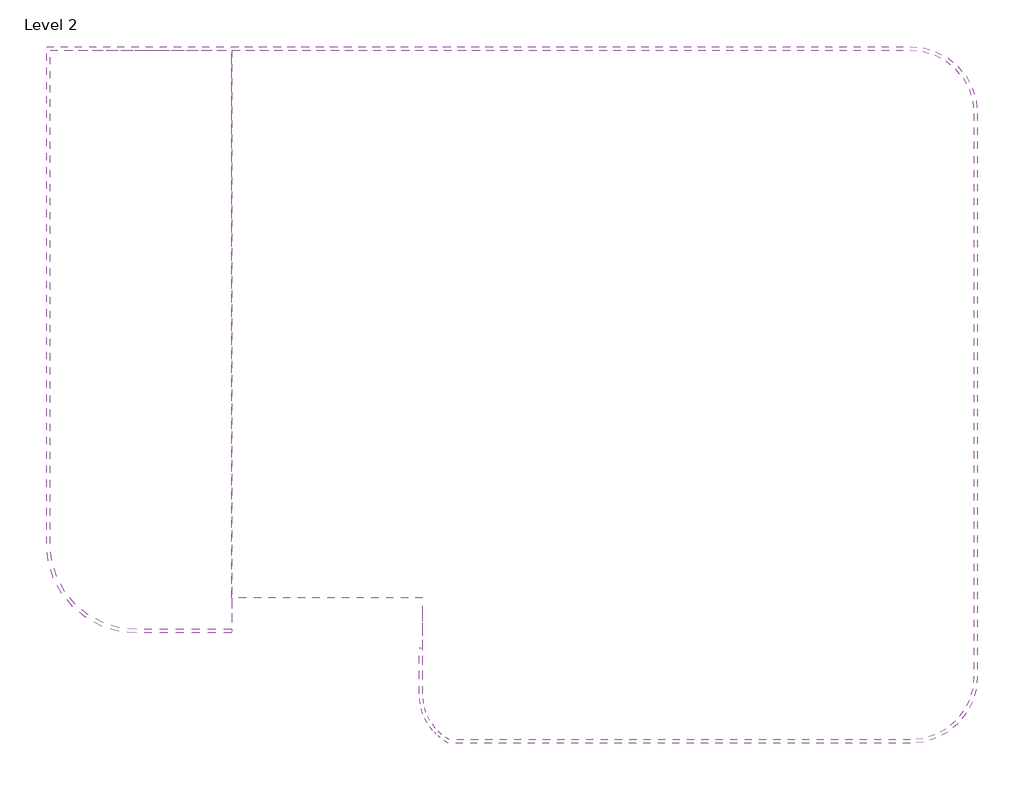
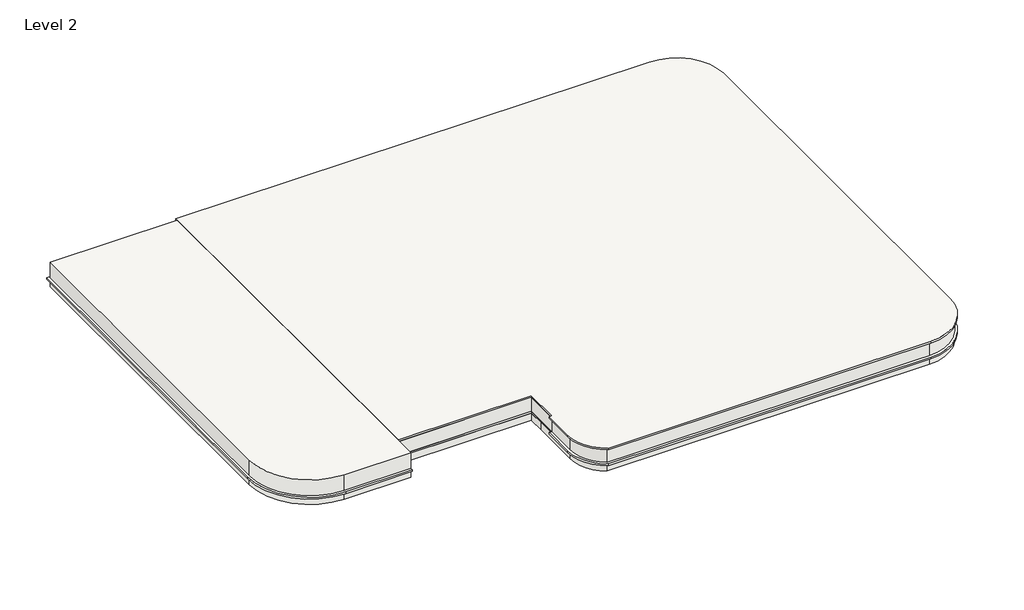
# One storey: 5 slabs.
"""IFC4 building model written with IfcOpenShell, lengths in millimetres."""

from ifc_helpers import new_model, si_unit, point, frame, frame_2d, origin, place, context, project, spatial, polyline, circle_curve, trimmed, segment, composite_curve, outline, extrude, element, save

model = new_model("IFC4")

# Units and contexts
model_context = context("Model", 3, world=origin())
ifc_project = project(units=[si_unit("LENGTHUNIT", "METRE", prefix="MILLI")], contexts=[model_context])

# Site, building, storey
site = spatial("IfcSite", under=ifc_project)
building = spatial("IfcBuilding", under=site)
storey = spatial("IfcBuildingStorey", under=building, Name="Level 2", Elevation=3048.0)

# Slabs
placement = place(None, origin())
element("IfcSlab", 1, ObjectType="Generic - 12\"", at=placement, inside=storey, context=model_context, shape_type="SweptSolid", body=[
    extrude(outline(composite_curve([segment(polyline([(-6917.636879, -5795.1908042), (-6917.636879, -3712.3908042), (-6917.636879, -3028.3602909), (-12404.036879, -3028.3602909), (-12404.036879, -3942.7602909), (-15147.236879, -3942.7602909)]), True, "CONTINUOUS"), segment(trimmed(circle_curve(frame_2d((-15147.236879, -1474.8121743)), 2467.9481165), [point((-15147.236879, -3942.7602909))], [point((-17615.1849955, -1474.8121743))], False, "CARTESIAN"), True, "CONTINUOUS"), segment(polyline([(-17615.1849955, -1474.8121743), (-17615.1849955, 12700.6437739), (7073.6150045, 12700.6437739)]), True, "CONTINUOUS"), segment(trimmed(circle_curve(frame_2d((7073.6150045, 10871.8437739)), 1828.8), [point((7073.6150045, 12700.6437739))], [point((8902.4150045, 10871.8437739))], False, "CARTESIAN"), True, "CONTINUOUS"), segment(polyline([(8902.4150045, 10871.8437739), (8902.4150045, -5282.5562261)]), True, "CONTINUOUS"), segment(trimmed(circle_curve(frame_2d((7073.6150045, -5282.5562261)), 1828.8), [point((8902.4150045, -5282.5562261))], [point((7073.6150045, -7111.3562261))], False, "CARTESIAN"), True, "CONTINUOUS"), segment(polyline([(7073.6150045, -7111.3562261), (-6155.636879, -7111.3562261)]), True, "CONTINUOUS"), segment(trimmed(circle_curve(frame_2d((-5399.9627203, -5795.1908042)), 1517.6741587), [point((-6155.636879, -7111.3562261))], [point((-6917.636879, -5795.1908042))], False, "CARTESIAN"), True, "CONTINUOUS")], self_intersect=False)), frame((0.0, 0.0, 4927.6), z_axis=(0.0, 0.0, 1.0), x_axis=(1.0, 0.0, 0.0)), (0.0, 0.0, 1.0), 304.8),
])
element("IfcSlab", 2, ObjectType="Generic - 2'", at=placement, inside=storey, context=model_context, shape_type="SweptSolid", body=[
    extrude(outline(composite_curve([segment(polyline([(-6917.636879, -4474.3908042), (-6917.636879, -3028.3602909), (-12404.036879, -3028.3602909), (-12404.036879, 12700.6437739), (7073.6150045, 12700.6437739)]), True, "CONTINUOUS"), segment(trimmed(circle_curve(frame_2d((7073.6150045, 10871.8437739)), 1828.8), [point((7073.6150045, 12700.6437739))], [point((8902.4150045, 10871.8437739))], False, "CARTESIAN"), True, "CONTINUOUS"), segment(polyline([(8902.4150045, 10871.8437739), (8902.4150045, -5282.5562261)]), True, "CONTINUOUS"), segment(trimmed(circle_curve(frame_2d((7073.6150045, -5282.5562261)), 1828.8), [point((8902.4150045, -5282.5562261))], [point((7073.6150045, -7111.3562261))], False, "CARTESIAN"), True, "CONTINUOUS"), segment(polyline([(7073.6150045, -7111.3562261), (-6155.636879, -7111.3562261)]), True, "CONTINUOUS"), segment(trimmed(circle_curve(frame_2d((-5399.9627203, -5795.1908042)), 1517.6741587), [point((-6155.636879, -7111.3562261))], [point((-6917.636879, -5795.1908042))], False, "CARTESIAN"), True, "CONTINUOUS"), segment(polyline([(-6917.636879, -5795.1908042), (-6917.636879, -4474.3908042)]), True, "CONTINUOUS")], self_intersect=False)), frame((0.0, 0.0, 5308.6), z_axis=(0.0, 0.0, 1.0), x_axis=(1.0, 0.0, 0.0)), (0.0, 0.0, 1.0), 609.6),
])
element("IfcSlab", 3, ObjectType="Generic - 2'5\"", at=placement, inside=storey, context=model_context, shape_type="SweptSolid", body=[
    extrude(outline(composite_curve([segment(polyline([(-17615.1849955, 12700.6437739), (-12404.036879, 12700.6437739), (-12404.036879, -3942.7602909), (-15147.236879, -3942.7602909)]), True, "CONTINUOUS"), segment(trimmed(circle_curve(frame_2d((-15147.236879, -1474.8121743)), 2467.9481165), [point((-15147.236879, -3942.7602909))], [point((-17615.1849955, -1474.8121743))], False, "CARTESIAN"), True, "CONTINUOUS"), segment(polyline([(-17615.1849955, -1474.8121743), (-17615.1849955, 12700.6437739)]), True, "CONTINUOUS")], self_intersect=False)), frame((0.0, 0.0, 5308.6), z_axis=(0.0, 0.0, 1.0), x_axis=(1.0, 0.0, 0.0)), (0.0, 0.0, 1.0), 685.8),
])
element("IfcSlab", 4, ObjectType="Generic - 3\"", at=placement, inside=storey, context=model_context, shape_type="SweptSolid", body=[
    extrude(outline(composite_curve([segment(polyline([(-6917.636879, -3028.3602909), (-12404.036879, -3028.3602909), (-12404.036879, -3942.7602909), (-12404.036879, -4044.3602909), (-15147.236879, -4044.3602909)]), True, "CONTINUOUS"), segment(trimmed(circle_curve(frame_2d((-15147.236879, -1474.8121743)), 2569.5481165), [point((-15147.236879, -4044.3602909))], [point((-17716.7849955, -1474.8121743))], False, "CARTESIAN"), True, "CONTINUOUS"), segment(polyline([(-17716.7849955, -1474.8121743), (-17716.7849955, 12802.2437739), (7073.6150045, 12802.2437739)]), True, "CONTINUOUS"), segment(trimmed(circle_curve(frame_2d((7073.6150045, 10871.8437739)), 1930.4), [point((7073.6150045, 12802.2437739))], [point((9004.0150045, 10871.8437739))], False, "CARTESIAN"), True, "CONTINUOUS"), segment(polyline([(9004.0150045, 10871.8437739), (9004.0150045, -5282.5562261)]), True, "CONTINUOUS"), segment(trimmed(circle_curve(frame_2d((7073.6150045, -5282.5562261)), 1930.4), [point((9004.0150045, -5282.5562261))], [point((7073.6150045, -7212.9562261))], False, "CARTESIAN"), True, "CONTINUOUS"), segment(polyline([(7073.6150045, -7212.9562261), (-6182.2606235, -7212.9562261)]), True, "CONTINUOUS"), segment(trimmed(circle_curve(frame_2d((-5399.9627203, -5795.1908042)), 1619.2741587), [point((-6182.2606235, -7212.9562261))], [point((-7019.236879, -5795.1908042))], False, "CARTESIAN"), True, "CONTINUOUS"), segment(polyline([(-7019.236879, -5795.1908042), (-7019.236879, -4474.3908042), (-6917.636879, -4474.3908042), (-6917.636879, -3028.3602909)]), True, "CONTINUOUS")], self_intersect=False)), frame((0.0, 0.0, 5232.4), z_axis=(0.0, 0.0, 1.0), x_axis=(1.0, 0.0, 0.0)), (0.0, 0.0, 1.0), 76.2),
])
element("IfcSlab", 5, ObjectType="Generic - 3\"", at=placement, inside=storey, context=model_context, shape_type="SweptSolid", body=[
    extrude(outline(composite_curve([segment(polyline([(-6917.636879, -3028.3602909), (-12404.036879, -3028.3602909), (-12404.036879, 12802.2437739), (7073.6150045, 12802.2437739)]), True, "CONTINUOUS"), segment(trimmed(circle_curve(frame_2d((7073.6150045, 10871.8437739)), 1930.4), [point((7073.6150045, 12802.2437739))], [point((9004.0150045, 10871.8437739))], False, "CARTESIAN"), True, "CONTINUOUS"), segment(polyline([(9004.0150045, 10871.8437739), (9004.0150045, -5282.5562261)]), True, "CONTINUOUS"), segment(trimmed(circle_curve(frame_2d((7073.6150045, -5282.5562261)), 1930.4), [point((9004.0150045, -5282.5562261))], [point((7073.6150045, -7212.9562261))], False, "CARTESIAN"), True, "CONTINUOUS"), segment(polyline([(7073.6150045, -7212.9562261), (-6182.2606235, -7212.9562261)]), True, "CONTINUOUS"), segment(trimmed(circle_curve(frame_2d((-5399.9627203, -5795.1908042)), 1619.2741587), [point((-6182.2606235, -7212.9562261))], [point((-7019.236879, -5795.1908042))], False, "CARTESIAN"), True, "CONTINUOUS"), segment(polyline([(-7019.236879, -5795.1908042), (-7019.236879, -4474.3908042), (-6917.636879, -4474.3908042), (-6917.636879, -3028.3602909)]), True, "CONTINUOUS")], self_intersect=False)), frame((0.0, 0.0, 5918.2), z_axis=(0.0, 0.0, 1.0), x_axis=(1.0, 0.0, 0.0)), (0.0, 0.0, 1.0), 76.2),
])

save(model, "model.ifc")

# Revit data of these elements
# Type "Generic - 12\""
#   Assembly Code = "B1010"
#   Function = 0
#   Layers, outside or top first: 1' - 0" "Parking Stripe" (function 1)
# Type "Generic - 2'"
#   Assembly Code = "B1010"
#   Function = 0
#   Layers, outside or top first: 2' - 0" "Parking Stripe" (function 1)
# Type "Generic - 2'5\""
#   Assembly Code = "B1010"
#   Function = 0
#   Layers, outside or top first: 2' - 3" "Parking Stripe" (function 1)
# Type "Generic - 3\""
#   Assembly Code = "B1010"
#   Function = 0
#   Layers, outside or top first: 0' - 3" "Rigid insulation" (function 1)
# Element 1 (IfcSlab, "Generic - 12\"")
#   built-in parameter 1001955 = -1.5708 (stored number, unit not read)
#   Height Offset From Level = 7' - 2"
#   Phase Created = New Construction
#   Materials on its faces: "Parking Stripe", "Door - Frame"
# Element 2 (IfcSlab, "Generic - 2'")
#   built-in parameter 1001955 = -1.5708 (stored number, unit not read)
#   Height Offset From Level = 9' - 5"
#   Phase Created = New Construction
#   Materials on its faces: "Parking Stripe"
# Element 3 (IfcSlab, "Generic - 2'5\"")
#   built-in parameter 1001955 = -1.5708 (stored number, unit not read)
#   Height Offset From Level = 9' - 8"
#   Phase Created = New Construction
#   Materials on its faces: "Parking Stripe", "Tile, Porcelain, 4in"
# Element 4 (IfcSlab, "Generic - 3\"")
#   Height Offset From Level = 7' - 5"
#   Phase Created = New Construction
#   Materials on its faces: "Rigid insulation"
# Element 5 (IfcSlab, "Generic - 3\"")
#   built-in parameter 1001955 = 1.5708 (stored number, unit not read)
#   Height Offset From Level = 9' - 8"
#   Phase Created = New Construction
#   Materials on its faces: "Rigid insulation", "Tile, Porcelain, 4in"
# Materials
#   "Parking Stripe": class "Paint", colour RGB 250 250 91, transparency 0, Cost = 0
#   "Rigid insulation": class "Generic", colour RGB 127 127 127, transparency 0, Description = "Rigid foam insulation board", Cost = 0
#   "Door - Frame": colour RGB 118 70 51, transparency 0, Cost = 0
#   "Tile, Porcelain, 4in": class "Generic", colour RGB 89 87 158, transparency 0, Description = "Porcelain tile, 4\", white", Cost = 0
